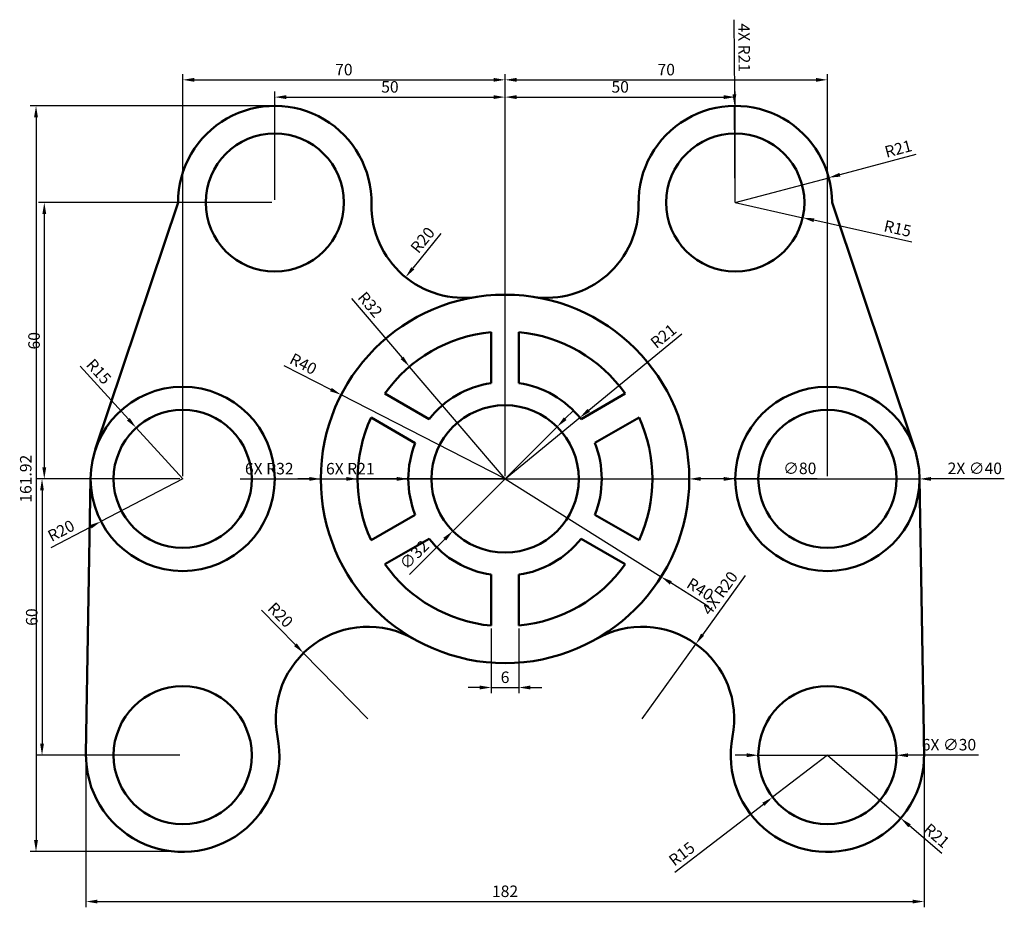
# Model space of a CAD drawing. Units: millimetres. Extents: x 2141 to 2355, y 1666 to 1858.
import ezdxf

# ---------------------------------------------------------------- set-up
doc = ezdxf.new("R2010")
doc.units = ezdxf.units.MM
doc.layers.add('M-DIMS', color=1, linetype='Continuous', lineweight=25)
doc.layers.add('M-OUTL', color=7, linetype='Continuous', lineweight=50)
doc.styles.get("Standard").update_dxf_attribs({"font": 'arial.ttf'})
doc.dimstyles.new('ISO-25', dxfattribs={"dimtxt": 2.5, "dimasz": 2.5, "dimexe": 1.25, "dimexo": 0.625, "dimtad": 1, "dimtxsty": 'Standard', "dimcen": 2.5, "dimadec": 0, "dimazin": 0, "dimtfac": 1, "dimtmove": 0, "dimatfit": 3, "dimfxl": 1, "dimarcsym": 0})

# ---------------------------------------------------------------- blocks, each defined once
blk = doc.blocks.new('*D1')
at = {"layer": 'Defpoints', "color": 0, "transparency": 16777216}
for p in [(2196.66, 1818.66), (2146.61, 1758.66), (2176.66, 1758.66)]:
    blk.add_point(p, dxfattribs=at)
at = {"layer": 'M-DIMS', "color": 0, "lineweight": -2, "transparency": 16777216}
for p, q in [((2196.03, 1818.66), (2145.36, 1818.66)), ((2146.61, 1816.16), (2146.61, 1761.16)), ((2176.03, 1758.66), (2145.36, 1758.66))]:
    blk.add_line(p, q, dxfattribs=at)
at = {"layer": 'M-DIMS', "color": 0, "transparency": 16777216}
for points in [[(2146.19, 1816.16), (2147.03, 1816.16), (2146.61, 1818.66)], [(2146.19, 1761.16), (2147.03, 1761.16), (2146.61, 1758.66)]]:
    blk.add_solid(points, dxfattribs=at)
at = {"layer": 'M-DIMS', "color": 0, "transparency": 16777216, "insert": (2144.71, 1788.66), "char_height": 2.5, "attachment_point": 5, "rotation": 90}
blk.add_mtext('60', dxfattribs=at)
blk = doc.blocks.new('*D2')
at = {"layer": 'Defpoints', "color": 0, "transparency": 16777216}
for p in [(2176.66, 1758.66), (2146.12, 1698.66), (2176.66, 1698.66)]:
    blk.add_point(p, dxfattribs=at)
at = {"layer": 'M-DIMS', "color": 0, "lineweight": -2, "transparency": 16777216}
for p, q in [((2176.03, 1758.66), (2144.87, 1758.66)), ((2146.12, 1756.16), (2146.12, 1701.16)), ((2176.03, 1698.66), (2144.87, 1698.66))]:
    blk.add_line(p, q, dxfattribs=at)
at = {"layer": 'M-DIMS', "color": 0, "transparency": 16777216}
for points in [[(2145.7, 1756.16), (2146.53, 1756.16), (2146.12, 1758.66)], [(2145.7, 1701.16), (2146.53, 1701.16), (2146.12, 1698.66)]]:
    blk.add_solid(points, dxfattribs=at)
at = {"layer": 'M-DIMS', "color": 0, "transparency": 16777216, "insert": (2144.21, 1728.66), "char_height": 2.5, "attachment_point": 5, "rotation": 90}
blk.add_mtext('60', dxfattribs=at)
blk = doc.blocks.new('*D3')
at = {"layer": 'Defpoints', "color": 0, "transparency": 16777216}
for p in [(2246.66, 1845.31), (2176.66, 1758.66), (2246.66, 1758.66)]:
    blk.add_point(p, dxfattribs=at)
at = {"layer": 'M-DIMS', "color": 0, "lineweight": -2, "transparency": 16777216}
for p, q in [((2176.66, 1759.29), (2176.66, 1846.56)), ((2179.16, 1845.31), (2244.16, 1845.31)), ((2246.66, 1759.29), (2246.66, 1846.56))]:
    blk.add_line(p, q, dxfattribs=at)
at = {"layer": 'M-DIMS', "color": 0, "transparency": 16777216}
for points in [[(2179.16, 1845.73), (2179.16, 1844.89), (2176.66, 1845.31)], [(2244.16, 1845.73), (2244.16, 1844.89), (2246.66, 1845.31)]]:
    blk.add_solid(points, dxfattribs=at)
at = {"layer": 'M-DIMS', "color": 0, "transparency": 16777216, "insert": (2211.66, 1847.21), "char_height": 2.5, "attachment_point": 5}
blk.add_mtext('70', dxfattribs=at)
blk = doc.blocks.new('*D4')
at = {"layer": 'Defpoints', "color": 0, "transparency": 16777216}
for p in [(2316.66, 1845.31), (2246.66, 1758.66), (2316.66, 1758.66)]:
    blk.add_point(p, dxfattribs=at)
at = {"layer": 'M-DIMS', "color": 0, "lineweight": -2, "transparency": 16777216}
for p, q in [((2246.66, 1759.29), (2246.66, 1846.56)), ((2249.16, 1845.31), (2314.16, 1845.31)), ((2316.66, 1759.29), (2316.66, 1846.56))]:
    blk.add_line(p, q, dxfattribs=at)
at = {"layer": 'M-DIMS', "color": 0, "transparency": 16777216}
for points in [[(2249.16, 1845.73), (2249.16, 1844.89), (2246.66, 1845.31)], [(2314.16, 1845.73), (2314.16, 1844.89), (2316.66, 1845.31)]]:
    blk.add_solid(points, dxfattribs=at)
at = {"layer": 'M-DIMS', "color": 0, "transparency": 16777216, "insert": (2281.66, 1847.21), "char_height": 2.5, "attachment_point": 5}
blk.add_mtext('70', dxfattribs=at)
blk = doc.blocks.new('*D5')
at = {"layer": 'Defpoints', "color": 0, "transparency": 16777216}
for p in [(2246.66, 1841.56), (2196.66, 1818.66), (2246.66, 1758.66)]:
    blk.add_point(p, dxfattribs=at)
at = {"layer": 'M-DIMS', "color": 0, "lineweight": -2, "transparency": 16777216}
for p, q in [((2196.66, 1819.29), (2196.66, 1842.81)), ((2199.16, 1841.56), (2244.16, 1841.56)), ((2246.66, 1759.29), (2246.66, 1842.81))]:
    blk.add_line(p, q, dxfattribs=at)
at = {"layer": 'M-DIMS', "color": 0, "transparency": 16777216}
for points in [[(2199.16, 1841.98), (2199.16, 1841.14), (2196.66, 1841.56)], [(2244.16, 1841.98), (2244.16, 1841.14), (2246.66, 1841.56)]]:
    blk.add_solid(points, dxfattribs=at)
at = {"layer": 'M-DIMS', "color": 0, "transparency": 16777216, "insert": (2221.66, 1843.46), "char_height": 2.5, "attachment_point": 5}
blk.add_mtext('50', dxfattribs=at)
blk = doc.blocks.new('*D6')
at = {"layer": 'Defpoints', "color": 0, "transparency": 16777216}
for p in [(2296.66, 1841.56), (2296.66, 1818.66), (2246.66, 1758.66)]:
    blk.add_point(p, dxfattribs=at)
at = {"layer": 'M-DIMS', "color": 0, "lineweight": -2, "transparency": 16777216}
for p, q in [((2246.66, 1759.29), (2246.66, 1842.81)), ((2249.16, 1841.56), (2294.16, 1841.56)), ((2296.66, 1819.29), (2296.66, 1842.81))]:
    blk.add_line(p, q, dxfattribs=at)
at = {"layer": 'M-DIMS', "color": 0, "transparency": 16777216}
for points in [[(2249.16, 1841.98), (2249.16, 1841.14), (2246.66, 1841.56)], [(2294.16, 1841.98), (2294.16, 1841.14), (2296.66, 1841.56)]]:
    blk.add_solid(points, dxfattribs=at)
at = {"layer": 'M-DIMS', "color": 0, "transparency": 16777216, "insert": (2271.66, 1843.46), "char_height": 2.5, "attachment_point": 5}
blk.add_mtext('50', dxfattribs=at)
blk = doc.blocks.new('*D7')
at = {"layer": 'Defpoints', "color": 0, "transparency": 16777216}
for p in [(2243.66, 1726.8), (2249.66, 1726.8), (2249.66, 1713.37)]:
    blk.add_point(p, dxfattribs=at)
at = {"layer": 'M-DIMS', "color": 0, "lineweight": -2, "transparency": 16777216}
for p, q in [((2243.66, 1726.18), (2243.66, 1712.12)), ((2249.66, 1726.18), (2249.66, 1712.12)), ((2241.16, 1713.37), (2238.66, 1713.37)), ((2243.66, 1713.37), (2249.66, 1713.37)), ((2252.16, 1713.37), (2254.66, 1713.37))]:
    blk.add_line(p, q, dxfattribs=at)
at = {"layer": 'M-DIMS', "color": 0, "transparency": 16777216}
for points in [[(2241.16, 1713.79), (2241.16, 1712.95), (2243.66, 1713.37)], [(2252.16, 1713.79), (2252.16, 1712.95), (2249.66, 1713.37)]]:
    blk.add_solid(points, dxfattribs=at)
at = {"layer": 'M-DIMS', "color": 0, "transparency": 16777216, "insert": (2246.66, 1715.27), "char_height": 2.5, "attachment_point": 5}
blk.add_mtext('6', dxfattribs=at)
blk = doc.blocks.new('*D8')
at = {"layer": 'Defpoints', "color": 0, "transparency": 16777216}
for p in [(2166.56, 1769.76), (2176.66, 1758.66)]:
    blk.add_point(p, dxfattribs=at)
at = {"layer": 'M-DIMS', "color": 0, "lineweight": -2, "transparency": 16777216}
for p, q in [((2154.37, 1783.14), (2164.88, 1771.6)), ((2176.66, 1758.66), (2166.56, 1769.76))]:
    blk.add_line(p, q, dxfattribs=at)
at = {"layer": 'M-DIMS', "color": 0, "transparency": 16777216}
blk.add_solid([(2165.18, 1771.88), (2164.57, 1771.32), (2166.56, 1769.76)], dxfattribs=at)
at = {"layer": 'M-DIMS', "color": 0, "transparency": 16777216, "insert": (2158.21, 1781.75), "char_height": 2.5, "attachment_point": 5, "rotation": 312.3151}
blk.add_mtext('R15', dxfattribs=at)
blk = doc.blocks.new('*D9')
at = {"layer": 'Defpoints', "color": 0, "transparency": 16777216}
for p in [(2176.66, 1758.66), (2158.92, 1749.42)]:
    blk.add_point(p, dxfattribs=at)
at = {"layer": 'M-DIMS', "color": 0, "lineweight": -2, "transparency": 16777216}
for p, q in [((2176.66, 1758.66), (2158.92, 1749.42)), ((2148.09, 1743.78), (2156.7, 1748.27))]:
    blk.add_line(p, q, dxfattribs=at)
at = {"layer": 'M-DIMS', "color": 0, "transparency": 16777216}
blk.add_solid([(2156.51, 1748.64), (2156.89, 1747.9), (2158.92, 1749.42)], dxfattribs=at)
at = {"layer": 'M-DIMS', "color": 0, "transparency": 16777216, "insert": (2150.41, 1747.13), "char_height": 2.5, "attachment_point": 5, "rotation": 27.5168}
blk.add_mtext('R20', dxfattribs=at)
blk = doc.blocks.new('*D10')
at = {"layer": 'Defpoints', "color": 0, "transparency": 16777216}
for p in [(2211.07, 1776.92), (2246.66, 1758.66)]:
    blk.add_point(p, dxfattribs=at)
at = {"layer": 'M-DIMS', "color": 0, "lineweight": -2, "transparency": 16777216}
for p, q in [((2198.63, 1783.3), (2208.84, 1778.06)), ((2246.66, 1758.66), (2211.07, 1776.92))]:
    blk.add_line(p, q, dxfattribs=at)
at = {"layer": 'M-DIMS', "color": 0, "transparency": 16777216}
blk.add_solid([(2209.03, 1778.43), (2208.65, 1777.69), (2211.07, 1776.92)], dxfattribs=at)
at = {"layer": 'M-DIMS', "color": 0, "transparency": 16777216, "insert": (2202.71, 1783.34), "char_height": 2.5, "attachment_point": 5, "rotation": 332.8442}
blk.add_mtext('R40', dxfattribs=at)
blk = doc.blocks.new('*D11')
at = {"layer": 'Defpoints', "color": 0, "transparency": 16777216}
for p in [(2225.92, 1783.03), (2246.66, 1758.66)]:
    blk.add_point(p, dxfattribs=at)
at = {"layer": 'M-DIMS', "color": 0, "lineweight": -2, "transparency": 16777216}
for p, q in [((2213.34, 1797.81), (2224.3, 1784.94)), ((2246.66, 1758.66), (2225.92, 1783.03))]:
    blk.add_line(p, q, dxfattribs=at)
at = {"layer": 'M-DIMS', "color": 0, "transparency": 16777216}
blk.add_solid([(2224.61, 1785.21), (2223.98, 1784.67), (2225.92, 1783.03)], dxfattribs=at)
at = {"layer": 'M-DIMS', "color": 0, "transparency": 16777216, "insert": (2217.12, 1796.3), "char_height": 2.5, "attachment_point": 5, "rotation": 310.4011}
blk.add_mtext('R32', dxfattribs=at)
blk = doc.blocks.new('*D12')
at = {"layer": 'Defpoints', "color": 0, "transparency": 16777216}
for p in [(2262.9, 1771.97), (2246.66, 1758.66)]:
    blk.add_point(p, dxfattribs=at)
at = {"layer": 'M-DIMS', "color": 0, "lineweight": -2, "transparency": 16777216}
for p, q in [((2285.04, 1790.1), (2264.84, 1773.55)), ((2246.66, 1758.66), (2262.9, 1771.97))]:
    blk.add_line(p, q, dxfattribs=at)
at = {"layer": 'M-DIMS', "color": 0, "transparency": 16777216}
blk.add_solid([(2264.57, 1773.88), (2265.1, 1773.23), (2262.9, 1771.97)], dxfattribs=at)
at = {"layer": 'M-DIMS', "color": 0, "transparency": 16777216, "insert": (2281.25, 1789.42), "char_height": 2.5, "attachment_point": 5, "rotation": 39.3156}
blk.add_mtext('R21', dxfattribs=at)
blk = doc.blocks.new('*D13')
at = {"layer": 'Defpoints', "color": 0, "transparency": 16777216}
for p in [(2246.66, 1758.66), (2280.54, 1737.41)]:
    blk.add_point(p, dxfattribs=at)
at = {"layer": 'M-DIMS', "color": 0, "lineweight": -2, "transparency": 16777216}
for p, q in [((2246.66, 1758.66), (2280.54, 1737.41)), ((2290.89, 1730.92), (2282.66, 1736.08))]:
    blk.add_line(p, q, dxfattribs=at)
at = {"layer": 'M-DIMS', "color": 0, "transparency": 16777216}
blk.add_solid([(2282.88, 1736.44), (2282.44, 1735.73), (2280.54, 1737.41)], dxfattribs=at)
at = {"layer": 'M-DIMS', "color": 0, "transparency": 16777216, "insert": (2288.85, 1734.45), "char_height": 2.5, "attachment_point": 5, "rotation": 327.9053}
blk.add_mtext('R40', dxfattribs=at)
blk = doc.blocks.new('*D14')
at = {"layer": 'Defpoints', "color": 0, "transparency": 16777216}
for p in [(2202.89, 1720.86), (2216.89, 1706.57)]:
    blk.add_point(p, dxfattribs=at)
at = {"layer": 'M-DIMS', "color": 0, "lineweight": -2, "transparency": 16777216}
for p, q in [((2193.79, 1730.15), (2201.14, 1722.64)), ((2216.89, 1706.57), (2202.89, 1720.86))]:
    blk.add_line(p, q, dxfattribs=at)
at = {"layer": 'M-DIMS', "color": 0, "transparency": 16777216}
blk.add_solid([(2201.44, 1722.94), (2200.85, 1722.35), (2202.89, 1720.86)], dxfattribs=at)
at = {"layer": 'M-DIMS', "color": 0, "transparency": 16777216, "insert": (2197.67, 1728.91), "char_height": 2.5, "attachment_point": 5, "rotation": 314.4018}
blk.add_mtext('R20', dxfattribs=at)
blk = doc.blocks.new('*D15')
at = {"layer": 'Defpoints', "color": 0, "transparency": 16777216}
for p in [(2237.65, 1817.98), (2225.06, 1802.45)]:
    blk.add_point(p, dxfattribs=at)
at = {"layer": 'M-DIMS', "color": 0, "lineweight": -2, "transparency": 16777216}
blk.add_line((2232.75, 1811.94), (2226.63, 1804.39), dxfattribs=at)
at = {"layer": 'M-DIMS', "color": 0, "transparency": 16777216}
blk.add_solid([(2226.31, 1804.65), (2226.95, 1804.13), (2225.06, 1802.45)], dxfattribs=at)
at = {"layer": 'M-DIMS', "color": 0, "transparency": 16777216, "insert": (2229, 1810.33), "char_height": 2.5, "attachment_point": 5, "rotation": 50.9651}
blk.add_mtext('R20', dxfattribs=at)
blk = doc.blocks.new('*D16')
at = {"layer": 'Defpoints', "color": 0, "transparency": 16777216}
for p in [(2316.95, 1824.06), (2296.66, 1818.66)]:
    blk.add_point(p, dxfattribs=at)
at = {"layer": 'M-DIMS', "color": 0, "lineweight": -2, "transparency": 16777216}
for p, q in [((2335.87, 1829.09), (2319.37, 1824.7)), ((2296.66, 1818.66), (2316.95, 1824.06))]:
    blk.add_line(p, q, dxfattribs=at)
at = {"layer": 'M-DIMS', "color": 0, "transparency": 16777216}
blk.add_solid([(2319.26, 1825.11), (2319.47, 1824.3), (2316.95, 1824.06)], dxfattribs=at)
at = {"layer": 'M-DIMS', "color": 0, "transparency": 16777216, "insert": (2332.13, 1830.04), "char_height": 2.5, "attachment_point": 5, "rotation": 14.8912}
blk.add_mtext('R21', dxfattribs=at)
blk = doc.blocks.new('*D17')
at = {"layer": 'Defpoints', "color": 0, "transparency": 16777216}
for p in [(2296.66, 1818.66), (2311.29, 1815.38)]:
    blk.add_point(p, dxfattribs=at)
at = {"layer": 'M-DIMS', "color": 0, "lineweight": -2, "transparency": 16777216}
for p, q in [((2296.66, 1818.66), (2311.29, 1815.38)), ((2334.96, 1810.06), (2313.73, 1814.83))]:
    blk.add_line(p, q, dxfattribs=at)
at = {"layer": 'M-DIMS', "color": 0, "transparency": 16777216}
blk.add_solid([(2313.82, 1815.24), (2313.64, 1814.42), (2311.29, 1815.38)], dxfattribs=at)
at = {"layer": 'M-DIMS', "color": 0, "transparency": 16777216, "insert": (2331.84, 1812.71), "char_height": 2.5, "attachment_point": 5, "rotation": 347.3457}
blk.add_mtext('R15', dxfattribs=at)
blk = doc.blocks.new('*D18')
at = {"layer": 'Defpoints', "color": 0, "transparency": 16777216}
for p in [(2316.66, 1698.66), (2304.75, 1689.54)]:
    blk.add_point(p, dxfattribs=at)
at = {"layer": 'M-DIMS', "color": 0, "lineweight": -2, "transparency": 16777216}
for p, q in [((2316.66, 1698.66), (2304.75, 1689.54)), ((2283.51, 1673.28), (2302.76, 1688.02))]:
    blk.add_line(p, q, dxfattribs=at)
at = {"layer": 'M-DIMS', "color": 0, "transparency": 16777216}
blk.add_solid([(2302.51, 1688.35), (2303.02, 1687.69), (2304.75, 1689.54)], dxfattribs=at)
at = {"layer": 'M-DIMS', "color": 0, "transparency": 16777216, "insert": (2285.23, 1676.99), "char_height": 2.5, "attachment_point": 5, "rotation": 37.4507}
blk.add_mtext('R15', dxfattribs=at)
blk = doc.blocks.new('*D19')
at = {"layer": 'Defpoints', "color": 0, "transparency": 16777216}
for p in [(2316.66, 1698.66), (2332.59, 1684.98)]:
    blk.add_point(p, dxfattribs=at)
at = {"layer": 'M-DIMS', "color": 0, "lineweight": -2, "transparency": 16777216}
for p, q in [((2316.66, 1698.66), (2332.59, 1684.98)), ((2341.5, 1677.33), (2334.49, 1683.35))]:
    blk.add_line(p, q, dxfattribs=at)
at = {"layer": 'M-DIMS', "color": 0, "transparency": 16777216}
blk.add_solid([(2334.76, 1683.67), (2334.21, 1683.04), (2332.59, 1684.98)], dxfattribs=at)
at = {"layer": 'M-DIMS', "color": 0, "transparency": 16777216, "insert": (2340.16, 1680.96), "char_height": 2.5, "attachment_point": 5, "rotation": 319.3458}
blk.add_mtext('R21', dxfattribs=at)
blk = doc.blocks.new('RADIAL-CUTOUT-R21-R32')
for p, q in [((23.09, 7.79), (23.09, 18.87)), ((9.59, 0), (0, 5.54))]:
    blk.add_line(p, q)
for radius, start, end in [(32, 95.3794, 144.6206), (21, 98.2132, 141.7868)]:
    blk.add_arc((26.09, -12.99), radius, start, end)
blk = doc.blocks.new('MOUNT-HOLE-D30')
blk.add_circle((15, 15), 15)
blk = doc.blocks.new('MOUNT-HOLE-D30-RIM-D40')
for radius in [20, 15]:
    blk.add_circle((20, 20), radius)
blk = doc.blocks.new('*D23')
at = {"layer": 'Defpoints', "color": 0, "transparency": 16777216}
for p in [(2155.66, 1699.01), (2337.65, 1699.01), (2337.65, 1666.9)]:
    blk.add_point(p, dxfattribs=at)
at = {"layer": 'M-DIMS', "color": 0, "lineweight": -2, "transparency": 16777216}
for p, q in [((2155.66, 1698.39), (2155.66, 1665.65)), ((2337.65, 1698.39), (2337.65, 1665.65)), ((2158.16, 1666.9), (2335.15, 1666.9))]:
    blk.add_line(p, q, dxfattribs=at)
at = {"layer": 'M-DIMS', "color": 0, "transparency": 16777216}
for points in [[(2158.16, 1667.31), (2158.16, 1666.48), (2155.66, 1666.9)], [(2335.15, 1667.31), (2335.15, 1666.48), (2337.65, 1666.9)]]:
    blk.add_solid(points, dxfattribs=at)
at = {"layer": 'M-DIMS', "color": 0, "transparency": 16777216, "insert": (2246.66, 1668.8), "char_height": 2.5, "attachment_point": 5}
blk.add_mtext('182', dxfattribs=at)
blk = doc.blocks.new('*D24')
at = {"layer": 'Defpoints', "color": 0, "transparency": 16777216}
for p in [(2196.83, 1839.66), (2144.81, 1677.75), (2178.52, 1677.75)]:
    blk.add_point(p, dxfattribs=at)
at = {"layer": 'M-DIMS', "color": 0, "lineweight": -2, "transparency": 16777216}
for p, q in [((2196.21, 1839.66), (2143.56, 1839.66)), ((2144.81, 1837.16), (2144.81, 1680.25)), ((2177.89, 1677.75), (2143.56, 1677.75))]:
    blk.add_line(p, q, dxfattribs=at)
at = {"layer": 'M-DIMS', "color": 0, "transparency": 16777216}
for points in [[(2144.39, 1837.16), (2145.23, 1837.16), (2144.81, 1839.66)], [(2144.39, 1680.25), (2145.23, 1680.25), (2144.81, 1677.75)]]:
    blk.add_solid(points, dxfattribs=at)
at = {"layer": 'M-DIMS', "color": 0, "transparency": 16777216, "insert": (2142.91, 1758.7), "char_height": 2.5, "attachment_point": 5, "rotation": 90}
blk.add_mtext('161.92', dxfattribs=at)
blk = doc.blocks.new('*D25')
at = {"layer": 'Defpoints', "color": 0, "transparency": 16777216}
for p in [(2301.66, 1698.66), (2331.66, 1698.66)]:
    blk.add_point(p, dxfattribs=at)
at = {"layer": 'M-DIMS', "color": 0, "lineweight": -2, "transparency": 16777216}
for p, q in [((2299.16, 1698.66), (2296.66, 1698.66)), ((2301.66, 1698.66), (2331.66, 1698.66)), ((2349.45, 1698.66), (2334.16, 1698.66))]:
    blk.add_line(p, q, dxfattribs=at)
at = {"layer": 'M-DIMS', "color": 0, "transparency": 16777216}
for points in [[(2299.16, 1699.08), (2299.16, 1698.25), (2301.66, 1698.66)], [(2334.16, 1699.08), (2334.16, 1698.25), (2331.66, 1698.66)]]:
    blk.add_solid(points, dxfattribs=at)
at = {"layer": 'M-DIMS', "color": 0, "transparency": 16777216, "insert": (2343.05, 1700.63), "char_height": 2.5, "attachment_point": 5, "rotation": 359.9984}
blk.add_mtext('6X ∅30', dxfattribs=at)
blk = doc.blocks.new('*D26')
at = {"layer": 'Defpoints', "color": 0, "transparency": 16777216}
for p in [(2296.66, 1758.66), (2336.66, 1758.66)]:
    blk.add_point(p, dxfattribs=at)
at = {"layer": 'M-DIMS', "color": 0, "lineweight": -2, "transparency": 16777216}
for p, q in [((2294.16, 1758.66), (2291.66, 1758.66)), ((2296.66, 1758.66), (2336.66, 1758.66)), ((2355.07, 1758.66), (2339.16, 1758.66))]:
    blk.add_line(p, q, dxfattribs=at)
at = {"layer": 'M-DIMS', "color": 0, "transparency": 16777216}
for points in [[(2294.16, 1759.08), (2294.16, 1758.25), (2296.66, 1758.66)], [(2339.16, 1759.08), (2339.16, 1758.25), (2336.66, 1758.66)]]:
    blk.add_solid(points, dxfattribs=at)
at = {"layer": 'M-DIMS', "color": 0, "transparency": 16777216, "insert": (2348.66, 1760.63), "char_height": 2.5, "attachment_point": 5, "rotation": 359.9988}
blk.add_mtext('2X ∅40', dxfattribs=at)
blk = doc.blocks.new('*D27')
at = {"layer": 'Defpoints', "color": 0, "transparency": 16777216}
for p in [(2257.97, 1769.98), (2235.34, 1747.35)]:
    blk.add_point(p, dxfattribs=at)
at = {"layer": 'M-DIMS', "color": 0, "lineweight": -2, "transparency": 16777216}
for p, q in [((2259.74, 1771.75), (2261.51, 1773.51)), ((2257.97, 1769.98), (2235.34, 1747.35)), ((2225.89, 1737.9), (2233.58, 1745.58))]:
    blk.add_line(p, q, dxfattribs=at)
at = {"layer": 'M-DIMS', "color": 0, "transparency": 16777216}
for points in [[(2259.44, 1772.04), (2260.03, 1771.45), (2257.97, 1769.98)], [(2233.28, 1745.88), (2233.87, 1745.29), (2235.34, 1747.35)]]:
    blk.add_solid(points, dxfattribs=at)
at = {"layer": 'M-DIMS', "color": 0, "transparency": 16777216, "insert": (2227.16, 1741.96), "char_height": 2.5, "attachment_point": 5, "rotation": 45.0008}
blk.add_mtext('∅32', dxfattribs=at)
blk = doc.blocks.new('*D28')
at = {"layer": 'Defpoints', "color": 0, "transparency": 16777216}
for p in [(2206.66, 1758.66), (2286.66, 1758.66)]:
    blk.add_point(p, dxfattribs=at)
at = {"layer": 'M-DIMS', "color": 0, "lineweight": -2, "transparency": 16777216}
for p, q in [((2204.16, 1758.66), (2201.66, 1758.66)), ((2206.66, 1758.66), (2286.66, 1758.66)), ((2314.43, 1758.66), (2289.16, 1758.66))]:
    blk.add_line(p, q, dxfattribs=at)
at = {"layer": 'M-DIMS', "color": 0, "transparency": 16777216}
for points in [[(2204.16, 1759.08), (2204.16, 1758.25), (2206.66, 1758.66)], [(2289.16, 1759.08), (2289.16, 1758.25), (2286.66, 1758.66)]]:
    blk.add_solid(points, dxfattribs=at)
at = {"layer": 'M-DIMS', "color": 0, "transparency": 16777216, "insert": (2310.66, 1760.63), "char_height": 2.5, "attachment_point": 5, "rotation": 359.9994}
blk.add_mtext('∅80', dxfattribs=at)
blk = doc.blocks.new('*D29')
at = {"layer": 'Defpoints', "color": 0, "transparency": 16777216}
for p in [(2296.48, 1839.66), (2296.66, 1818.66)]:
    blk.add_point(p, dxfattribs=at)
at = {"layer": 'M-DIMS', "color": 0, "lineweight": -2, "transparency": 16777216}
for p, q in [((2296.33, 1858.37), (2296.46, 1842.16)), ((2296.66, 1818.66), (2296.48, 1839.66))]:
    blk.add_line(p, q, dxfattribs=at)
at = {"layer": 'M-DIMS', "color": 0, "transparency": 16777216}
blk.add_solid([(2296.88, 1842.17), (2296.05, 1842.16), (2296.48, 1839.66)], dxfattribs=at)
at = {"layer": 'M-DIMS', "color": 0, "transparency": 16777216, "insert": (2298.26, 1852.28), "char_height": 2.5, "attachment_point": 5, "rotation": 270.475}
blk.add_mtext('4X R21', dxfattribs=at)
blk = doc.blocks.new('*D30')
at = {"layer": 'Defpoints', "color": 0, "transparency": 16777216}
for p in [(2288.09, 1722.81), (2276.43, 1706.57)]:
    blk.add_point(p, dxfattribs=at)
at = {"layer": 'M-DIMS', "color": 0, "lineweight": -2, "transparency": 16777216}
for p, q in [((2298.79, 1737.71), (2289.55, 1724.84)), ((2276.43, 1706.57), (2288.09, 1722.81))]:
    blk.add_line(p, q, dxfattribs=at)
at = {"layer": 'M-DIMS', "color": 0, "transparency": 16777216}
blk.add_solid([(2289.21, 1725.09), (2289.89, 1724.6), (2288.09, 1722.81)], dxfattribs=at)
at = {"layer": 'M-DIMS', "color": 0, "transparency": 16777216, "insert": (2293.55, 1733.67), "char_height": 2.5, "attachment_point": 5, "rotation": 54.315}
blk.add_mtext('4X R20', dxfattribs=at)
blk = doc.blocks.new('*D31')
at = {"layer": 'Defpoints', "color": 0, "transparency": 16777216}
for p in [(2214.66, 1758.66), (2246.66, 1758.66)]:
    blk.add_point(p, dxfattribs=at)
at = {"layer": 'M-DIMS', "color": 0, "lineweight": -2, "transparency": 16777216}
for p, q in [((2189.17, 1758.66), (2212.16, 1758.66)), ((2246.66, 1758.66), (2214.66, 1758.66))]:
    blk.add_line(p, q, dxfattribs=at)
at = {"layer": 'M-DIMS', "color": 0, "transparency": 16777216}
blk.add_solid([(2212.16, 1759.08), (2212.16, 1758.25), (2214.66, 1758.66)], dxfattribs=at)
at = {"layer": 'M-DIMS', "color": 0, "transparency": 16777216, "insert": (2195.46, 1760.57), "char_height": 2.5, "attachment_point": 5, "rotation": 0.0008}
blk.add_mtext('6X R32', dxfattribs=at)
blk = doc.blocks.new('*D32')
at = {"layer": 'Defpoints', "color": 0, "transparency": 16777216}
for p in [(2225.66, 1758.66), (2246.66, 1758.66)]:
    blk.add_point(p, dxfattribs=at)
at = {"layer": 'M-DIMS', "color": 0, "lineweight": -2, "transparency": 16777216}
for p, q in [((2206.99, 1758.66), (2223.16, 1758.66)), ((2246.66, 1758.66), (2225.66, 1758.66))]:
    blk.add_line(p, q, dxfattribs=at)
at = {"layer": 'M-DIMS', "color": 0, "transparency": 16777216}
blk.add_solid([(2223.16, 1759.08), (2223.16, 1758.25), (2225.66, 1758.66)], dxfattribs=at)
at = {"layer": 'M-DIMS', "color": 0, "transparency": 16777216, "insert": (2213.06, 1760.56), "char_height": 2.5, "attachment_point": 5}
blk.add_mtext('6X R21', dxfattribs=at)

msp = doc.modelspace()

# ---------------------------------------------------------------- linework, layer by layer
at = {"layer": 'M-OUTL'}
for p, q in [((2175.657, 1818.663), (2157.692, 1765.014)), ((2317.657, 1818.663), (2335.622, 1765.014)), ((2156.657, 1758.663), (2155.66, 1699.014)), ((2336.657, 1758.663), (2337.654, 1699.014))]:
    msp.add_line(p, q, dxfattribs=at)
for radius in [40, 16]:
    msp.add_circle((2246.657, 1758.663), radius, dxfattribs=at)
for centre, radius, start, end in [((2196.657, 1818.663), 21, 359.05011, 180), ((2296.657, 1818.663), 21, 0, 180.94989), ((2237.651, 1817.984), 20, 179.05011, 278.63237), ((2255.663, 1817.984), 20, 261.36763, 0.94989), ((2216.888, 1706.569), 20, 60.25385, 191.11804), ((2276.427, 1706.569), 20, 348.88196, 119.74615), ((2176.657, 1698.663), 21, 179.04236, 11.11804), ((2316.657, 1698.663), 21, 168.88196, 0.95764)]:
    msp.add_arc(centre, radius, start, end, dxfattribs=at)

# ---------------------------------------------------------------- block references
for name, p in [('MOUNT-HOLE-D30', (2181.657, 1803.663)), ('MOUNT-HOLE-D30', (2281.657, 1803.663)), ('RADIAL-CUTOUT-R21-R32', (2220.566, 1771.654)), ('MOUNT-HOLE-D30-RIM-D40', (2156.657, 1738.663)), ('MOUNT-HOLE-D30-RIM-D40', (2296.657, 1738.663)), ('MOUNT-HOLE-D30', (2161.657, 1683.663)), ('MOUNT-HOLE-D30', (2301.657, 1683.663))]:
    msp.add_blockref(name, p, dxfattribs=at)
for p, rotation in [((2244.862, 1787.754), 299.9999999999985), ((2270.953, 1774.764), 240.0000000000009), ((2222.361, 1742.563), 59.99999999999826), ((2248.452, 1729.573), 119.9999999999982), ((2272.748, 1745.673), 180)]:
    msp.add_blockref('RADIAL-CUTOUT-R21-R32', p, dxfattribs=dict(at, rotation=rotation))

# ---------------------------------------------------------------- dimensions: what is measured, and where the dimension line sits
at = {"layer": 'M-DIMS'}
for center, mpoint, text, picture, middle in [((2296.657, 1818.663), (2296.483, 1839.663), '4X <>', '*D29', (2296.379, 1852.262)), ((2246.657, 1758.663), (2214.657, 1758.663), '6X <>', '*D31', (2195.457, 1758.663)), ((2246.657, 1758.663), (2225.657, 1758.663), '6X <>', '*D32', (2213.057, 1758.663)), ((2276.427, 1706.569), (2288.093, 1722.814), '4X <>', '*D30', (2295.093, 1732.561))]:
    dim = msp.add_radius_dim(center=center, mpoint=mpoint, text=text, dimstyle='ISO-25', override={"dimdec": 0, "dimlfac": 1, "dimrnd": 0, "dimzin": 0, "dimdsep": 46, "dimlunit": 2}, dxfattribs=at)
    dim.commit()
    dim.dimension.update_dxf_attribs({"geometry": picture, "text_midpoint": middle, "dimtype": 164})
for base, p1, p2, override, picture, middle in [((2246.657, 1845.311), (2176.657, 1758.663), (2246.657, 1758.663), {"dimclrd": 0, "dimclre": 0, "dimclrt": 0}, '*D3', (2211.657, 1847.213)), ((2316.657, 1845.311), (2246.657, 1758.663), (2316.657, 1758.663), {"dimclrd": 0, "dimclre": 0, "dimclrt": 0}, '*D4', (2281.657, 1847.213)), ((2246.657, 1841.561), (2196.657, 1818.663), (2246.657, 1758.663), {"dimclrd": 0, "dimclre": 0, "dimclrt": 0}, '*D5', (2221.657, 1843.463)), ((2296.657, 1841.561), (2246.657, 1758.663), (2296.657, 1818.663), {"dimclrd": 0, "dimclre": 0, "dimclrt": 0}, '*D6', (2271.657, 1843.463)), ((2249.657, 1713.369), (2243.657, 1726.804), (2249.657, 1726.804), {"dimclrd": 0, "dimclre": 0, "dimclrt": 0}, '*D7', (2246.657, 1715.27)), ((2337.654, 1666.896), (2155.66, 1699.014), (2337.654, 1699.014), {"dimdec": 0, "dimlfac": 1, "dimrnd": 0, "dimzin": 0, "dimdsep": 46, "dimlunit": 2}, '*D23', (2246.657, 1668.797))]:
    dim = msp.add_linear_dim(base=base, p1=p1, p2=p2, dimstyle='ISO-25', override=override, dxfattribs=at)
    dim.commit()
    dim.dimension.update_dxf_attribs({"geometry": picture, "text_midpoint": middle})
for base, p1, p2, override, picture, middle in [((2144.81, 1677.746), (2196.831, 1839.663), (2178.517, 1677.746), {"dimdec": 2, "dimlfac": 1, "dimrnd": 0, "dimzin": 0, "dimdsep": 46, "dimlunit": 2}, '*D24', (2142.909, 1758.704)), ((2146.61, 1758.663), (2196.657, 1818.663), (2176.657, 1758.663), {"dimclrd": 0, "dimclre": 0, "dimclrt": 0}, '*D1', (2144.708, 1788.663)), ((2146.116, 1698.663), (2176.657, 1758.663), (2176.657, 1698.663), {"dimclrd": 0, "dimclre": 0, "dimclrt": 0}, '*D2', (2144.215, 1728.663))]:
    dim = msp.add_linear_dim(base=base, p1=p1, p2=p2, angle=90, dimstyle='ISO-25', override=override, dxfattribs=at)
    dim.commit()
    dim.dimension.update_dxf_attribs({"geometry": picture, "text_midpoint": middle})
for center, mpoint, picture, middle in [((2296.657, 1818.663), (2316.952, 1824.06), '*D16', (2332.61, 1828.224)), ((2237.651, 1817.984), (2225.056, 1802.448), '*D15', (2230.477, 1809.135)), ((2296.657, 1818.663), (2311.293, 1815.377), '*D17', (2331.425, 1810.857)), ((2246.657, 1758.663), (2225.917, 1783.032), '*D11', (2215.672, 1795.07)), ((2246.657, 1758.663), (2262.904, 1771.969), '*D12', (2282.437, 1787.965)), ((2246.657, 1758.663), (2211.066, 1776.92), '*D10', (2201.845, 1781.65)), ((2176.657, 1758.663), (2166.559, 1769.755), '*D8', (2156.808, 1780.466)), ((2216.888, 1706.569), (2202.894, 1720.859), '*D14', (2196.314, 1727.577)), ((2316.657, 1698.663), (2304.749, 1689.542), '*D18', (2286.388, 1675.478))]:
    dim = msp.add_radius_dim(center=center, mpoint=mpoint, dimstyle='ISO-25', override={"dimclrd": 0, "dimclre": 0, "dimclrt": 0}, dxfattribs=at)
    dim.commit()
    dim.dimension.update_dxf_attribs({"geometry": picture, "text_midpoint": middle, "dimtype": 164})
for p1, p2, picture, middle in [((2257.971, 1769.977), (2235.344, 1747.35), '*D27', (2228.555, 1740.561)), ((2206.657, 1758.664), (2286.657, 1758.663), '*D28', (2310.657, 1758.663))]:
    dim = msp.add_diameter_dim_2p(p1=p1, p2=p2, dimstyle='ISO-25', override={"dimdec": 0, "dimlfac": 1, "dimrnd": 0, "dimzin": 0, "dimdsep": 46, "dimlunit": 2}, dxfattribs=at)
    dim.commit()
    dim.dimension.update_dxf_attribs({"geometry": picture, "text_midpoint": middle, "dimtype": 163})
for p1, p2, text, picture, middle in [((2296.657, 1758.664), (2336.657, 1758.663), '2X <>', '*D26', (2348.657, 1758.663)), ((2301.657, 1698.664), (2331.657, 1698.663), '6X <>', '*D25', (2343.055, 1698.663))]:
    dim = msp.add_diameter_dim_2p(p1=p1, p2=p2, text=text, dimstyle='ISO-25', override={"dimdec": 0, "dimlfac": 1, "dimrnd": 0, "dimzin": 0, "dimdsep": 46, "dimlunit": 2}, dxfattribs=at)
    dim.commit()
    dim.dimension.update_dxf_attribs({"geometry": picture, "text_midpoint": middle, "dimtype": 163})
for center, mpoint, picture, middle in [((2176.657, 1758.663), (2158.92, 1749.423), '*D9', (2150.407, 1747.133)), ((2246.657, 1758.663), (2280.544, 1737.411), '*D13', (2288.846, 1734.448)), ((2316.657, 1698.663), (2332.589, 1684.982), '*D19', (2340.164, 1680.955))]:
    dim = msp.add_radius_dim(center=center, mpoint=mpoint, dimstyle='ISO-25', override={"dimclrd": 0, "dimclre": 0, "dimclrt": 0}, dxfattribs=at)
    dim.commit()
    dim.dimension.update_dxf_attribs({"geometry": picture, "text_midpoint": middle})

doc.saveas('drawing.dxf')
